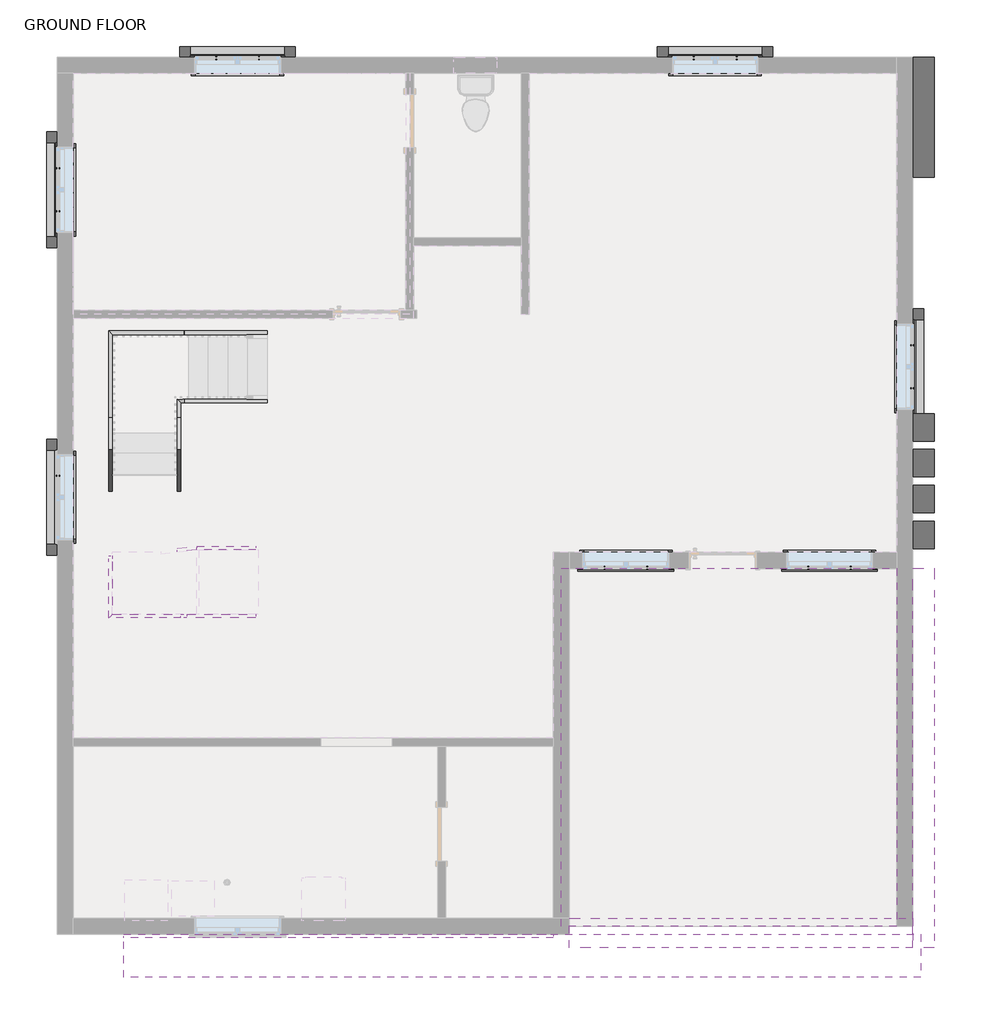
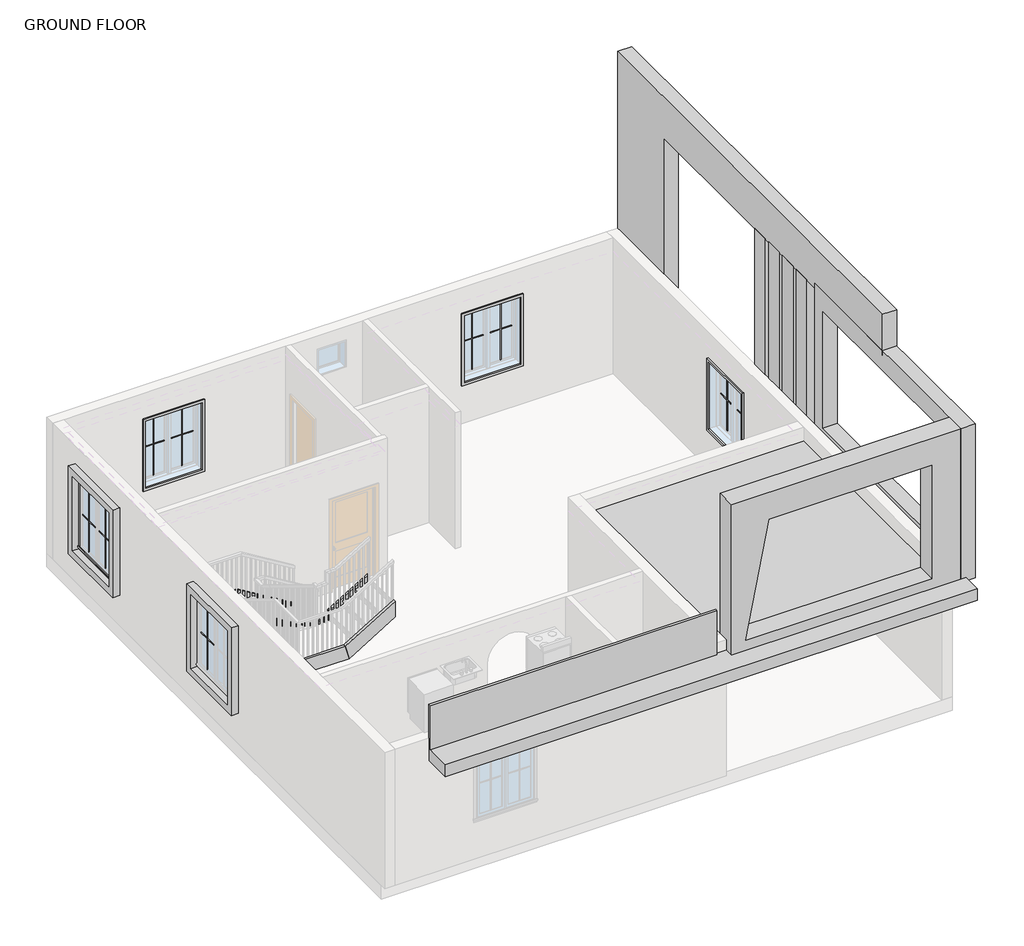
# One storey, part 4 of 4: 38 proxies, 12 members.
"""IFC4 building model written with IfcOpenShell, lengths in millimetres."""

from ifc_helpers import new_model, si_unit, frame, origin, place, context, project, spatial, polyline, outline, extrude, faceted_brep, transform, mapped, element, save
from components import generic_models_12_generic_models_12_6289c3a4, generic_models_16_generic_models_16_40d4eb7f, generic_models_17_generic_models_17_71cdcc77, generic_models_18_generic_models_18_24b474a2, generic_models_23_generic_models_23_7b700280, generic_models_24_generic_models_24_dfffe260, generic_models_25_generic_models_25_fd65dc18, generic_models_5_generic_models_1_92fab196, generic_models_6_generic_models_6_33fdfef5, generic_models_7_generic_models_7_aecf1bf8, generic_models_9_generic_models_9_3f232281, muntin_pattern_2x2_muntin_pattern_2x2_6dad3731, muntin_pattern_2x2_muntin_pattern_2x2_a30a3345, trim_window_exterior_flat_with_sill_92b9b949, trim_window_interior_flat_picture_frame_3bb882cf

model = new_model("IFC4")

# Units and contexts
model_context = context("Model", 3, world=origin())
ifc_project = project(units=[si_unit("LENGTHUNIT", "METRE", prefix="MILLI")], contexts=[model_context])

# Site, building, storey
site = spatial("IfcSite", under=ifc_project)
building = spatial("IfcBuilding", under=site)
storey = spatial("IfcBuildingStorey", under=building, Name="GROUND FLOOR", Elevation=304.8)

# Proxies
placement = place(None, origin())
generic_models_12_generic_models_12_shape = generic_models_12_generic_models_12_6289c3a4(model_context)
element("IfcBuildingElementProxy", 1, Name="Generic Models 12 : Generic Models 12", ObjectType="Generic Models 12 : Generic Models 12", at=placement, inside=storey, context=model_context, shape_type="MappedRepresentation", body=[
    mapped(generic_models_12_generic_models_12_shape, transform((0.0, 0.0, 0.0), x_axis=(1.0, 0.0, 0.0), y_axis=(0.0, 1.0, 0.0), z_axis=(0.0, 0.0, 1.0))),
])
generic_models_16_generic_models_16_shape = generic_models_16_generic_models_16_40d4eb7f(model_context)
element("IfcBuildingElementProxy", 2, Name="Generic Models 16 : Generic Models 16", ObjectType="Generic Models 16 : Generic Models 16", at=placement, inside=storey, context=model_context, shape_type="MappedRepresentation", body=[
    mapped(generic_models_16_generic_models_16_shape, transform((0.0, 0.0, 0.0), x_axis=(1.0, 0.0, 0.0), y_axis=(0.0, 1.0, 0.0), z_axis=(0.0, 0.0, 1.0))),
])
generic_models_17_generic_models_17_shape = generic_models_17_generic_models_17_71cdcc77(model_context)
element("IfcBuildingElementProxy", 3, Name="Generic Models 17 : Generic Models 17", ObjectType="Generic Models 17 : Generic Models 17", at=placement, inside=storey, context=model_context, shape_type="MappedRepresentation", body=[
    mapped(generic_models_17_generic_models_17_shape, transform((0.0, 0.0, 0.0), x_axis=(1.0, 0.0, 0.0), y_axis=(0.0, 1.0, 0.0), z_axis=(0.0, 0.0, 1.0))),
])
generic_models_18_generic_models_18_shape = generic_models_18_generic_models_18_24b474a2(model_context)
element("IfcBuildingElementProxy", 4, Name="Generic Models 20 : Generic Models 18", ObjectType="Generic Models 20 : Generic Models 18", at=placement, inside=storey, context=model_context, shape_type="MappedRepresentation", body=[
    mapped(generic_models_18_generic_models_18_shape, transform((0.0, -4352.925, -3048.0), x_axis=(1.0, 0.0, 0.0), y_axis=(0.0, 1.0, 0.0), z_axis=(0.0, 0.0, 1.0))),
])
element("IfcBuildingElementProxy", 5, Name="Generic Models 21 : Generic Models 18", ObjectType="Generic Models 21 : Generic Models 18", at=placement, inside=storey, context=model_context, shape_type="MappedRepresentation", body=[
    mapped(generic_models_18_generic_models_18_shape, transform((0.0, 0.0, -3048.0), x_axis=(1.0, 0.0, 0.0), y_axis=(0.0, 1.0, 0.0), z_axis=(0.0, 0.0, 1.0))),
])
generic_models_23_generic_models_23_shape = generic_models_23_generic_models_23_7b700280(model_context)
element("IfcBuildingElementProxy", 6, Name="Generic Models 23 : Generic Models 23", ObjectType="Generic Models 23 : Generic Models 23", at=placement, inside=storey, context=model_context, shape_type="MappedRepresentation", body=[
    mapped(generic_models_23_generic_models_23_shape, transform((0.0, 0.0, 0.0), x_axis=(1.0, 0.0, 0.0), y_axis=(0.0, 1.0, 0.0), z_axis=(0.0, 0.0, 1.0))),
])
generic_models_24_generic_models_24_shape = generic_models_24_generic_models_24_dfffe260(model_context)
element("IfcBuildingElementProxy", 7, Name="Generic Models 24 : Generic Models 24", ObjectType="Generic Models 24 : Generic Models 24", at=placement, inside=storey, context=model_context, shape_type="MappedRepresentation", body=[
    mapped(generic_models_24_generic_models_24_shape, transform((0.0, 0.0, 0.0), x_axis=(1.0, 0.0, 0.0), y_axis=(0.0, 1.0, 0.0), z_axis=(0.0, 0.0, 1.0))),
])
generic_models_25_generic_models_25_shape = generic_models_25_generic_models_25_fd65dc18(model_context)
element("IfcBuildingElementProxy", 8, Name="Generic Models 25 : Generic Models 25", ObjectType="Generic Models 25 : Generic Models 25", at=placement, inside=storey, context=model_context, shape_type="MappedRepresentation", body=[
    mapped(generic_models_25_generic_models_25_shape, transform((0.0, -914.4, 0.0), x_axis=(1.0, 0.0, 0.0), y_axis=(0.0, 1.0, 0.0), z_axis=(0.0, 0.0, 1.0))),
])
generic_models_5_generic_models_1_shape = generic_models_5_generic_models_1_92fab196(model_context)
element("IfcBuildingElementProxy", 9, Name="Generic Models 5 : Generic Models 1", ObjectType="Generic Models 5 : Generic Models 1", at=placement, inside=storey, context=model_context, shape_type="MappedRepresentation", body=[
    mapped(generic_models_5_generic_models_1_shape, transform((0.0, 0.0, -3276.6), x_axis=(1.0, 0.0, 0.0), y_axis=(0.0, 1.0, 0.0), z_axis=(0.0, 0.0, 1.0))),
])
generic_models_6_generic_models_6_shape = generic_models_6_generic_models_6_33fdfef5(model_context)
element("IfcBuildingElementProxy", 10, Name="Generic Models 6 : Generic Models 6", ObjectType="Generic Models 6 : Generic Models 6", at=placement, inside=storey, context=model_context, shape_type="MappedRepresentation", body=[
    mapped(generic_models_6_generic_models_6_shape, transform((0.0, 0.0, 0.0), x_axis=(1.0, 0.0, 0.0), y_axis=(0.0, 1.0, 0.0), z_axis=(0.0, 0.0, 1.0))),
])
generic_models_7_generic_models_7_shape = generic_models_7_generic_models_7_aecf1bf8(model_context)
element("IfcBuildingElementProxy", 11, Name="Generic Models 7 : Generic Models 7", ObjectType="Generic Models 7 : Generic Models 7", at=placement, inside=storey, context=model_context, shape_type="MappedRepresentation", body=[
    mapped(generic_models_7_generic_models_7_shape, transform((0.0, 0.0, 0.0), x_axis=(1.0, 0.0, 0.0), y_axis=(0.0, 1.0, 0.0), z_axis=(0.0, 0.0, 1.0))),
])
generic_models_9_generic_models_9_shape = generic_models_9_generic_models_9_3f232281(model_context)
element("IfcBuildingElementProxy", 12, Name="Generic Models 9 : Generic Models 9", ObjectType="Generic Models 9 : Generic Models 9", at=placement, inside=storey, context=model_context, shape_type="MappedRepresentation", body=[
    mapped(generic_models_9_generic_models_9_shape, transform((0.0, 0.0, 0.0), x_axis=(1.0, 0.0, 0.0), y_axis=(0.0, 1.0, 0.0), z_axis=(0.0, 0.0, 1.0))),
])
muntin_pattern_2x2_muntin_pattern_2x2_shape = muntin_pattern_2x2_muntin_pattern_2x2_6dad3731(model_context)
element("IfcBuildingElementProxy", 13, Name="Muntin Pattern_2x2 : Muntin Pattern_2x2", ObjectType="Muntin Pattern_2x2 : Muntin Pattern_2x2", at=placement, inside=storey, context=model_context, shape_type="MappedRepresentation", body=[
    mapped(muntin_pattern_2x2_muntin_pattern_2x2_shape, transform((-811.7461008, -2258.8594117, 1289.05), x_axis=(-1.0, 0.0, 0.0), y_axis=(0.0, -1.0, 0.0), z_axis=(0.0, 0.0, 1.0))),
])
element("IfcBuildingElementProxy", 14, Name="Muntin Pattern_2x2 : Muntin Pattern_2x2", ObjectType="Muntin Pattern_2x2 : Muntin Pattern_2x2", at=placement, inside=storey, context=model_context, shape_type="MappedRepresentation", body=[
    mapped(muntin_pattern_2x2_muntin_pattern_2x2_shape, transform((-3694.6461008, -2258.8594117, 1289.05), x_axis=(-1.0, 0.0, 0.0), y_axis=(0.0, -1.0, 0.0), z_axis=(0.0, 0.0, 1.0))),
])
element("IfcBuildingElementProxy", 15, Name="Muntin Pattern_2x2 : Muntin Pattern_2x2", ObjectType="Muntin Pattern_2x2 : Muntin Pattern_2x2", at=placement, inside=storey, context=model_context, shape_type="MappedRepresentation", body=[
    mapped(muntin_pattern_2x2_muntin_pattern_2x2_shape, transform((56.6163992, 892.3280883, 1289.05), x_axis=(0.0, -1.0, 0.0), y_axis=(1.0, 0.0, 0.0), z_axis=(0.0, 0.0, 1.0))),
])
element("IfcBuildingElementProxy", 16, Name="Muntin Pattern_2x2 : Muntin Pattern_2x2", ObjectType="Muntin Pattern_2x2 : Muntin Pattern_2x2", at=placement, inside=storey, context=model_context, shape_type="MappedRepresentation", body=[
    mapped(muntin_pattern_2x2_muntin_pattern_2x2_shape, transform((-9800.1711008, 4961.0905883, 1289.05), x_axis=(1.0, 0.0, 0.0), y_axis=(0.0, 1.0, 0.0), z_axis=(0.0, 0.0, 1.0))),
])
element("IfcBuildingElementProxy", 17, Name="Muntin Pattern_2x2 : Muntin Pattern_2x2", ObjectType="Muntin Pattern_2x2 : Muntin Pattern_2x2", at=placement, inside=storey, context=model_context, shape_type="MappedRepresentation", body=[
    mapped(muntin_pattern_2x2_muntin_pattern_2x2_shape, transform((-12040.1336008, 2790.9780883, 1289.05), x_axis=(0.0, 1.0, 0.0), y_axis=(-1.0, 0.0, 0.0), z_axis=(0.0, 0.0, 1.0))),
])
element("IfcBuildingElementProxy", 18, Name="Muntin Pattern_2x2 : Muntin Pattern_2x2", ObjectType="Muntin Pattern_2x2 : Muntin Pattern_2x2", at=placement, inside=storey, context=model_context, shape_type="MappedRepresentation", body=[
    mapped(muntin_pattern_2x2_muntin_pattern_2x2_shape, transform((-3037.4211008, 4961.0905883, 1289.05), x_axis=(1.0, 0.0, 0.0), y_axis=(0.0, 1.0, 0.0), z_axis=(0.0, 0.0, 1.0))),
])
muntin_pattern_2x2_muntin_pattern_2x2_2_shape = muntin_pattern_2x2_muntin_pattern_2x2_a30a3345(model_context)
element("IfcBuildingElementProxy", 19, Name="Muntin Pattern_2x2 : Muntin Pattern_2x2", ObjectType="Muntin Pattern_2x2 : Muntin Pattern_2x2", at=placement, inside=storey, context=model_context, shape_type="MappedRepresentation", body=[
    mapped(muntin_pattern_2x2_muntin_pattern_2x2_2_shape, transform((-1418.1711008, -2258.8594117, 1289.05), x_axis=(1.0, 0.0, 0.0), y_axis=(0.0, 1.0, 0.0), z_axis=(0.0, 0.0, 1.0))),
])
element("IfcBuildingElementProxy", 20, Name="Muntin Pattern_2x2 : Muntin Pattern_2x2", ObjectType="Muntin Pattern_2x2 : Muntin Pattern_2x2", at=placement, inside=storey, context=model_context, shape_type="MappedRepresentation", body=[
    mapped(muntin_pattern_2x2_muntin_pattern_2x2_2_shape, transform((-4301.0711008, -2258.8594117, 1289.05), x_axis=(1.0, 0.0, 0.0), y_axis=(0.0, 1.0, 0.0), z_axis=(0.0, 0.0, 1.0))),
])
element("IfcBuildingElementProxy", 21, Name="Muntin Pattern_2x2 : Muntin Pattern_2x2", ObjectType="Muntin Pattern_2x2 : Muntin Pattern_2x2", at=placement, inside=storey, context=model_context, shape_type="MappedRepresentation", body=[
    mapped(muntin_pattern_2x2_muntin_pattern_2x2_2_shape, transform((56.6163992, 285.9030883, 1289.05), x_axis=(0.0, 1.0, 0.0), y_axis=(-1.0, 0.0, 0.0), z_axis=(0.0, 0.0, 1.0))),
])
element("IfcBuildingElementProxy", 22, Name="Muntin Pattern_2x2 : Muntin Pattern_2x2", ObjectType="Muntin Pattern_2x2 : Muntin Pattern_2x2", at=placement, inside=storey, context=model_context, shape_type="MappedRepresentation", body=[
    mapped(muntin_pattern_2x2_muntin_pattern_2x2_2_shape, transform((-9193.7461008, 4961.0905883, 1289.05), x_axis=(-1.0, 0.0, 0.0), y_axis=(0.0, -1.0, 0.0), z_axis=(0.0, 0.0, 1.0))),
])
element("IfcBuildingElementProxy", 23, Name="Muntin Pattern_2x2 : Muntin Pattern_2x2", ObjectType="Muntin Pattern_2x2 : Muntin Pattern_2x2", at=placement, inside=storey, context=model_context, shape_type="MappedRepresentation", body=[
    mapped(muntin_pattern_2x2_muntin_pattern_2x2_2_shape, transform((-12040.1336008, 3397.4030883, 1289.05), x_axis=(0.0, -1.0, 0.0), y_axis=(1.0, 0.0, 0.0), z_axis=(0.0, 0.0, 1.0))),
])
element("IfcBuildingElementProxy", 24, Name="Muntin Pattern_2x2 : Muntin Pattern_2x2", ObjectType="Muntin Pattern_2x2 : Muntin Pattern_2x2", at=placement, inside=storey, context=model_context, shape_type="MappedRepresentation", body=[
    mapped(muntin_pattern_2x2_muntin_pattern_2x2_2_shape, transform((-12040.1336008, -955.5219117, 1289.05), x_axis=(0.0, -1.0, 0.0), y_axis=(1.0, 0.0, 0.0), z_axis=(0.0, 0.0, 1.0))),
])
element("IfcBuildingElementProxy", 25, Name="Muntin Pattern_2x2 : Muntin Pattern_2x2", ObjectType="Muntin Pattern_2x2 : Muntin Pattern_2x2", at=placement, inside=storey, context=model_context, shape_type="MappedRepresentation", body=[
    mapped(muntin_pattern_2x2_muntin_pattern_2x2_2_shape, transform((-2430.9961008, 4961.0905883, 1289.05), x_axis=(-1.0, 0.0, 0.0), y_axis=(0.0, -1.0, 0.0), z_axis=(0.0, 0.0, 1.0))),
])
trim_window_exterior_flat_with_sill_shape = trim_window_exterior_flat_with_sill_92b9b949(model_context)
element("IfcBuildingElementProxy", 26, Name="Trim-Window-Exterior-Flat : with Sill", ObjectType="Trim-Window-Exterior-Flat : with Sill", at=placement, inside=storey, context=model_context, shape_type="MappedRepresentation", body=[
    mapped(trim_window_exterior_flat_with_sill_shape, transform((-1114.9586008, -2268.3844117, 2743.2), x_axis=(1.0, 0.0, 0.0), y_axis=(0.0, 0.0, 1.0), z_axis=(0.0, -1.0, 0.0))),
])
element("IfcBuildingElementProxy", 27, Name="Trim-Window-Exterior-Flat : with Sill", ObjectType="Trim-Window-Exterior-Flat : with Sill", at=placement, inside=storey, context=model_context, shape_type="MappedRepresentation", body=[
    mapped(trim_window_exterior_flat_with_sill_shape, transform((-3997.8586008, -2268.3844117, 2743.2), x_axis=(1.0, 0.0, 0.0), y_axis=(0.0, 0.0, 1.0), z_axis=(0.0, -1.0, 0.0))),
])
element("IfcBuildingElementProxy", 28, Name="Trim-Window-Exterior-Flat : with Sill", ObjectType="Trim-Window-Exterior-Flat : with Sill", at=placement, inside=storey, context=model_context, shape_type="MappedRepresentation", body=[
    mapped(trim_window_exterior_flat_with_sill_shape, transform((66.1413992, 589.1155883, 2743.2), x_axis=(0.0, 1.0, 0.0), y_axis=(0.0, 0.0, 1.0), z_axis=(1.0, 0.0, 0.0))),
])
element("IfcBuildingElementProxy", 29, Name="Trim-Window-Exterior-Flat : with Sill", ObjectType="Trim-Window-Exterior-Flat : with Sill", at=placement, inside=storey, context=model_context, shape_type="MappedRepresentation", body=[
    mapped(trim_window_exterior_flat_with_sill_shape, transform((-9496.9586008, 4970.6155883, 2743.2), x_axis=(-1.0, 0.0, 0.0), y_axis=(0.0, 0.0, 1.0), z_axis=(0.0, 1.0, 0.0))),
])
element("IfcBuildingElementProxy", 30, Name="Trim-Window-Exterior-Flat : with Sill", ObjectType="Trim-Window-Exterior-Flat : with Sill", at=placement, inside=storey, context=model_context, shape_type="MappedRepresentation", body=[
    mapped(trim_window_exterior_flat_with_sill_shape, transform((-12049.6586008, 3094.1905883, 2743.2), x_axis=(0.0, -1.0, 0.0), y_axis=(0.0, 0.0, 1.0), z_axis=(-1.0, 0.0, 0.0))),
])
element("IfcBuildingElementProxy", 31, Name="Trim-Window-Exterior-Flat : with Sill", ObjectType="Trim-Window-Exterior-Flat : with Sill", at=placement, inside=storey, context=model_context, shape_type="MappedRepresentation", body=[
    mapped(trim_window_exterior_flat_with_sill_shape, transform((-2734.2086008, 4970.6155883, 2743.2), x_axis=(-1.0, 0.0, 0.0), y_axis=(0.0, 0.0, 1.0), z_axis=(0.0, 1.0, 0.0))),
])
trim_window_interior_flat_picture_frame_shape = trim_window_interior_flat_picture_frame_3bb882cf(model_context)
element("IfcBuildingElementProxy", 32, Name="Trim-Window-Interior-Flat : Picture Frame", ObjectType="Trim-Window-Interior-Flat : Picture Frame", at=placement, inside=storey, context=model_context, shape_type="MappedRepresentation", body=[
    mapped(trim_window_interior_flat_picture_frame_shape, transform((-1114.9586008, -2039.7844117, 2743.2), x_axis=(-1.0, 0.0, 0.0), y_axis=(0.0, 0.0, 1.0), z_axis=(0.0, 1.0, 0.0))),
])
element("IfcBuildingElementProxy", 33, Name="Trim-Window-Interior-Flat : Picture Frame", ObjectType="Trim-Window-Interior-Flat : Picture Frame", at=placement, inside=storey, context=model_context, shape_type="MappedRepresentation", body=[
    mapped(trim_window_interior_flat_picture_frame_shape, transform((-3997.8586008, -2039.7844117, 2743.2), x_axis=(-1.0, 0.0, 0.0), y_axis=(0.0, 0.0, 1.0), z_axis=(0.0, 1.0, 0.0))),
])
element("IfcBuildingElementProxy", 34, Name="Trim-Window-Interior-Flat : Picture Frame", ObjectType="Trim-Window-Interior-Flat : Picture Frame", at=placement, inside=storey, context=model_context, shape_type="MappedRepresentation", body=[
    mapped(trim_window_interior_flat_picture_frame_shape, transform((-162.4586008, 589.1155883, 2743.2), x_axis=(0.0, -1.0, 0.0), y_axis=(0.0, 0.0, 1.0), z_axis=(-1.0, 0.0, 0.0))),
])
element("IfcBuildingElementProxy", 35, Name="Trim-Window-Interior-Flat : Picture Frame", ObjectType="Trim-Window-Interior-Flat : Picture Frame", at=placement, inside=storey, context=model_context, shape_type="MappedRepresentation", body=[
    mapped(trim_window_interior_flat_picture_frame_shape, transform((-9496.9586008, 4742.0155883, 2743.2), x_axis=(1.0, 0.0, 0.0), y_axis=(0.0, 0.0, 1.0), z_axis=(0.0, -1.0, 0.0))),
])
element("IfcBuildingElementProxy", 36, Name="Trim-Window-Interior-Flat : Picture Frame", ObjectType="Trim-Window-Interior-Flat : Picture Frame", at=placement, inside=storey, context=model_context, shape_type="MappedRepresentation", body=[
    mapped(trim_window_interior_flat_picture_frame_shape, transform((-11821.0586008, 3094.1905883, 2743.2), x_axis=(0.0, 1.0, 0.0), y_axis=(0.0, 0.0, 1.0), z_axis=(1.0, 0.0, 0.0))),
])
element("IfcBuildingElementProxy", 37, Name="Trim-Window-Interior-Flat : Picture Frame", ObjectType="Trim-Window-Interior-Flat : Picture Frame", at=placement, inside=storey, context=model_context, shape_type="MappedRepresentation", body=[
    mapped(trim_window_interior_flat_picture_frame_shape, transform((-11821.0586008, -1258.7344117, 2743.2), x_axis=(0.0, 1.0, 0.0), y_axis=(0.0, 0.0, 1.0), z_axis=(1.0, 0.0, 0.0))),
])
element("IfcBuildingElementProxy", 38, Name="Trim-Window-Interior-Flat : Picture Frame", ObjectType="Trim-Window-Interior-Flat : Picture Frame", at=placement, inside=storey, context=model_context, shape_type="MappedRepresentation", body=[
    mapped(trim_window_interior_flat_picture_frame_shape, transform((-2734.2086008, 4742.0155883, 2743.2), x_axis=(1.0, 0.0, 0.0), y_axis=(0.0, 0.0, 1.0), z_axis=(0.0, -1.0, 0.0))),
])

# Members
element("IfcMember", 39, ObjectType="Stringer - 2\" Width", at=placement, inside=storey, context=model_context, shape_type="SweptSolid", body=[
    extrude(outline(polyline([(304.8, -9079.7156858), (516.914512, -9079.7156858), (1227.6666667, -10252.4567411), (922.8666667, -10337.6111976), (304.8, -9317.8011976), (304.8, -9079.7156858)])), frame((0.0, 79.9115003, 0.0), z_axis=(0.0, 1.0, 0.0), x_axis=(0.0, 0.0, 1.0)), (0.0, 0.0, 1.0), 50.8),
])
element("IfcMember", 40, ObjectType="Stringer - 2\" Width", at=placement, inside=storey, context=model_context, shape_type="SweptSolid", body=[
    extrude(outline(polyline([(304.8, -9079.7156858), (516.914512, -9079.7156858), (1227.6666667, -10252.4567411), (922.8666667, -10337.6111976), (304.8, -9317.8011976), (304.8, -9079.7156858)])), frame((0.0, 1045.1115003, 0.0), z_axis=(0.0, 1.0, 0.0), x_axis=(0.0, 0.0, 1.0)), (0.0, 0.0, 1.0), 50.8),
])
element("IfcMember", 41, ObjectType="Stringer - 2\" Width", at=placement, inside=storey, context=model_context, shape_type="Brep", body=[
    faceted_brep([(-10302.9522729, -132.1404207, 1227.6666667), (-10353.7522729, -132.1404207, 1227.6666667), (-10353.7522729, -1981.6853298, 2348.6029752), (-10302.9522729, -1976.0280655, 2345.1743302), (-10302.9522729, -217.2948772, 922.8666667), (-10302.9522729, -1976.0280655, 1988.7655687), (-10353.7522729, -217.2948772, 922.8666667), (-10353.7522729, -1981.6853298, 1992.1942137)], [[[0, 1, 2, 3]], [[4, 0, 3, 5]], [[6, 4, 5, 7]], [[1, 6, 7, 2]], [[1, 0, 4, 6]], [[2, 7, 5, 3]]]),
])
element("IfcMember", 42, ObjectType="Stringer - 2\" Width", at=placement, inside=storey, context=model_context, shape_type="SweptSolid", body=[
    extrude(outline(polyline([(-132.1404207, 1227.6666667), (-217.2948772, 922.8666667), (-2173.0948772, 2108.2), (-2087.9404207, 2413.0), (-132.1404207, 1227.6666667)])), frame((-11318.9522729, 0.0, 0.0), z_axis=(1.0, 0.0, 0.0), x_axis=(0.0, 1.0, 0.0)), (0.0, 0.0, 1.0), 50.8),
])
element("IfcMember", 43, ObjectType="Stringer - 2\" Width", at=placement, inside=storey, context=model_context, shape_type="Brep", body=[
    faceted_brep([(-10353.7522729, -132.1404207, 1227.6666667), (-10302.9522729, -132.1404207, 1227.6666667), (-10302.9522729, 79.9115003, 1227.6666667), (-10353.7522729, 130.7115003, 1227.6666667), (-10353.7522729, -217.2948772, 922.8666667), (-10353.7522729, 130.7115003, 922.8666667), (-10302.9522729, -217.2948772, 922.8666667), (-10302.9522729, 79.9115003, 922.8666667)], [[[0, 1, 2, 3]], [[4, 0, 3, 5]], [[6, 4, 5, 7]], [[1, 6, 7, 2]], [[1, 0, 4, 6]], [[2, 7, 5, 3]]]),
])
element("IfcMember", 44, ObjectType="Stringer - 2\" Width", at=placement, inside=storey, context=model_context, shape_type="Brep", body=[
    faceted_brep([(-10252.4567411, 1045.1115003, 1227.6666667), (-10252.4567411, 1095.9115003, 1227.6666667), (-11318.9522729, 1095.9115003, 1227.6666667), (-11268.1522729, 1045.1115003, 1227.6666667), (-10337.6111976, 1045.1115003, 922.8666667), (-11268.1522729, 1045.1115003, 922.8666667), (-10337.6111976, 1095.9115003, 922.8666667), (-11318.9522729, 1095.9115003, 922.8666667)], [[[0, 1, 2, 3]], [[4, 0, 3, 5]], [[6, 4, 5, 7]], [[1, 6, 7, 2]], [[1, 0, 4, 6]], [[2, 7, 5, 3]]]),
])
element("IfcMember", 45, ObjectType="Stringer - 2\" Width", at=placement, inside=storey, context=model_context, shape_type="Brep", body=[
    faceted_brep([(-11268.1522729, 1045.1115003, 1227.6666667), (-11318.9522729, 1095.9115003, 1227.6666667), (-11318.9522729, -132.1404207, 1227.6666667), (-11268.1522729, -132.1404207, 1227.6666667), (-11268.1522729, 1045.1115003, 922.8666667), (-11268.1522729, -217.2948772, 922.8666667), (-11318.9522729, 1095.9115003, 922.8666667), (-11318.9522729, -217.2948772, 922.8666667)], [[[0, 1, 2, 3]], [[4, 0, 3, 5]], [[6, 4, 5, 7]], [[1, 6, 7, 2]], [[1, 0, 4, 6]], [[2, 7, 5, 3]]]),
])
element("IfcMember", 46, ObjectType="Stringer - 2\" Width", at=placement, inside=storey, context=model_context, shape_type="SweptSolid", body=[
    extrude(outline(polyline([(2548.914512, -10074.3522729), (2192.5057504, -10074.3522729), (2700.5057504, -9236.1522729), (3056.914512, -9236.1522729), (2548.914512, -10074.3522729)])), frame((0.0, -2001.6844117, 0.0), z_axis=(0.0, 1.0, 0.0), x_axis=(0.0, 0.0, 1.0)), (0.0, 0.0, 1.0), 50.8),
])
element("IfcMember", 47, ObjectType="Stringer - 2\" Width", at=placement, inside=storey, context=model_context, shape_type="SweptSolid", body=[
    extrude(outline(polyline([(2413.0, -10298.6112176), (2108.2, -10213.4567611), (2700.5057504, -9236.1522729), (3056.914512, -9236.1522729), (2413.0, -10298.6112176)])), frame((0.0, -2966.8844117, 0.0), z_axis=(0.0, 1.0, 0.0), x_axis=(0.0, 0.0, 1.0)), (0.0, 0.0, 1.0), 50.8),
])
element("IfcMember", 48, ObjectType="Stringer - 2\" Width", at=placement, inside=storey, context=model_context, shape_type="SweptSolid", body=[
    extrude(outline(polyline([(-10074.3522729, -1950.570376), (-10074.3522729, -2001.6844117), (-10353.7522729, -2032.7993654), (-10353.7522729, -1981.6853298), (-10074.3522729, -1950.570376)])), frame((0.0, 0.0, 2108.2), z_axis=(0.0, 0.0, 1.0), x_axis=(1.0, 0.0, 0.0)), (0.0, 0.0, 1.0), 304.8),
])
element("IfcMember", 49, ObjectType="Stringer - 2\" Width", at=placement, inside=storey, context=model_context, shape_type="Brep", body=[
    faceted_brep([(-11268.1522729, -2087.9404207, 2413.0), (-11318.9522729, -2087.9404207, 2413.0), (-11318.9522729, -2966.8844117, 2413.0), (-11268.1522729, -2916.0844117, 2413.0), (-11268.1522729, -2173.0948772, 2108.2), (-11268.1522729, -2916.0844117, 2108.2), (-11318.9522729, -2173.0948772, 2108.2), (-11318.9522729, -2966.8844117, 2108.2)], [[[0, 1, 2, 3]], [[4, 0, 3, 5]], [[6, 4, 5, 7]], [[1, 6, 7, 2]], [[1, 0, 4, 6]], [[2, 7, 5, 3]]]),
])
element("IfcMember", 50, ObjectType="Stringer - 2\" Width", at=placement, inside=storey, context=model_context, shape_type="Brep", body=[
    faceted_brep([(-11268.1522729, -2916.0844117, 2413.0), (-11318.9522729, -2966.8844117, 2413.0), (-10298.6112176, -2966.8844117, 2413.0), (-10298.6112176, -2916.0844117, 2413.0), (-11268.1522729, -2916.0844117, 2108.2), (-10213.4567611, -2916.0844117, 2108.2), (-11318.9522729, -2966.8844117, 2108.2), (-10213.4567611, -2966.8844117, 2108.2)], [[[0, 1, 2, 3]], [[4, 0, 3, 5]], [[6, 4, 5, 7]], [[1, 6, 7, 2]], [[1, 0, 4, 6]], [[2, 7, 5, 3]]]),
])

save(model, "model.ifc")

# Revit data of these elements
# Type "Muntin Pattern_2x2 : Muntin Pattern_2x2"
#   Width [instance default] = 4' - 0"
#   Thickness = 0' - 0 1/2"
#   Height [instance default] = 4' - 0"
#   Distance = 0' - 0 3/4"
#   Interior Material [instance default] = none
#   Exterior Material [instance default] = none
#   Default Elevation = 0
# Type "Trim-Window-Exterior-Flat : with Sill"
#   Trim Width = 0' - 2 1/4"
#   Trim Thickness_Picture Frame = 0' - 1 1/4"
#   Trim Thickness_with Sill = 0' - 0 3/4"
#   Sill Thickness = 0' - 1 1/4"
#   Opening Width [instance default] = 2' - 0"
#   Opening Height [instance default] = 3' - 0"
#   Default Elevation = 4' - 0"
#   Sill = yes
#   Picture Frame = no
#   Trim Material [instance default] = none
# Type "Trim-Window-Interior-Flat : Picture Frame"
#   Trim Thickness_Picture Frame = 0' - 1 1/4"
#   Trim Width = 0' - 2 1/4"
#   Trim Thickness_with Sill = 0' - 0 3/4"
#   Sill Thickness = 0' - 1 1/4"
#   Opening Width [instance default] = 2' - 0"
#   Opening Height [instance default] = 3' - 0"
#   Default Elevation = 4' - 0"
#   Sill = no
#   Picture Frame = yes
#   Trim Material [instance default] = none
# Element 1 (IfcBuildingElementProxy, "Generic Models 12 : Generic Models 12")
#   Phase Created = New Construction
#   Materials on its faces: "feature frame"
# Element 2 (IfcBuildingElementProxy, "Generic Models 16 : Generic Models 16")
#   Phase Created = New Construction
#   Materials on its faces: "feature frame"
# Element 3 (IfcBuildingElementProxy, "Generic Models 17 : Generic Models 17")
#   Phase Created = New Construction
#   Materials on its faces: "feature frame"
# Element 4 (IfcBuildingElementProxy, "Generic Models 20 : Generic Models 18")
#   Phase Created = New Construction
#   Materials on its faces: "feature frame"
# Element 5 (IfcBuildingElementProxy, "Generic Models 21 : Generic Models 18")
#   Phase Created = New Construction
#   Materials on its faces: "feature frame"
# Element 6 (IfcBuildingElementProxy, "Generic Models 23 : Generic Models 23")
#   Phase Created = New Construction
#   Materials on its faces: "SAND STONE BEIGE CLADDING"
# Element 7 (IfcBuildingElementProxy, "Generic Models 24 : Generic Models 24")
#   Phase Created = New Construction
#   Materials on its faces: "OFF WHITE COLOUR"
# Element 8 (IfcBuildingElementProxy, "Generic Models 25 : Generic Models 25")
#   Phase Created = New Construction
#   Materials on its faces: "feature frame"
# Element 9 (IfcBuildingElementProxy, "Generic Models 5 : Generic Models 1")
#   Phase Created = New Construction
#   Materials on its faces: "Clad - White"
# Element 10 (IfcBuildingElementProxy, "Generic Models 6 : Generic Models 6")
#   Phase Created = New Construction
#   Materials on its faces: "feature frame"
# Element 11 (IfcBuildingElementProxy, "Generic Models 7 : Generic Models 7")
#   Phase Created = New Construction
#   Materials on its faces: "feature frame"
# Element 12 (IfcBuildingElementProxy, "Generic Models 9 : Generic Models 9")
#   Phase Created = New Construction
#   Materials on its faces: "wood ceiling"
# Elements 13, 14, 15, 16, 17, 18, 19, 20, 21, 22, 23, 24, 25 (IfcBuildingElementProxy, "Muntin Pattern_2x2 : Muntin Pattern_2x2")
#   Width = 1' - 6 5/8"
#   Height = 4' - 6 1/2"
#   Interior Material = Wood - Stained
#   Exterior Material = BLACK MATERIAL
#   Phase Created = New Construction
#   Materials on its faces: "BLACK MATERIAL", "Wood - Stained"
# Elements 26, 27, 28, 29, 30, 31 (IfcBuildingElementProxy, "Trim-Window-Exterior-Flat : with Sill")
#   Opening Width = 4' - 0"
#   Opening Height = 5' - 0"
#   Trim Material = BLACK MATERIAL
#   Phase Created = New Construction
#   Materials on its faces: "BLACK MATERIAL"
# Elements 32, 33, 34, 35, 36, 37, 38 (IfcBuildingElementProxy, "Trim-Window-Interior-Flat : Picture Frame")
#   Opening Width = 4' - 0"
#   Opening Height = 5' - 0"
#   Trim Material = Wood - Stained
#   Phase Created = New Construction
#   Materials on its faces: "Wood - Stained"
# Elements 39, 40, 41, 42, 43, 44, 45, 46, 47, 48, 49, 50 (IfcMember, "Stringer - 2\" Width")
#   Phase Created = New Construction
# Materials
#   "feature frame": class "Generic", colour RGB 120 120 120, transparency 0, Cost = 0
#   "SAND STONE BEIGE CLADDING": class "Generic", colour RGB 120 120 120, transparency 0, Cost = 0
#   "OFF WHITE COLOUR": class "Generic", colour RGB 120 120 120, transparency 0, Cost = 0
#   "Clad - White": class "Wood", colour RGB 242 242 238, transparency 0, Cost = 0
#   "wood ceiling": class "Generic", colour RGB 120 120 120, transparency 0, Cost = 0
#   "BLACK MATERIAL": class "Generic", colour RGB 120 120 120, transparency 0, Cost = 0
#   "Wood - Stained": class "Wood", colour RGB 224 178 126, transparency 0, Cost = 0
